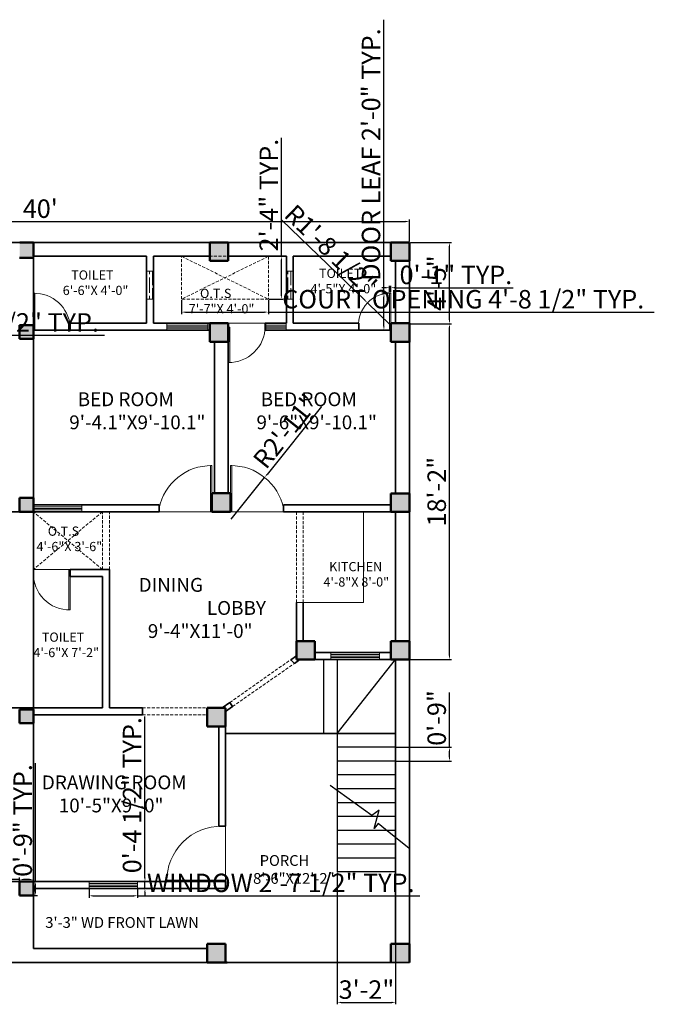
# Model space of a CAD drawing. Units: inches. Extents: x 2499 to 3266, y 1908 to 2597.
# Tile 2 of 2: x 2854 to 3266, y 1956 to 2597. Entities that reach past the tile are written whole.
import ezdxf

# ---------------------------------------------------------------- set-up
doc = ezdxf.new("R2010")
doc.units = ezdxf.units.IN
doc.linetypes.add('JIS_02_2.0', pattern=[3, 2, -1])
for name, color, linetype, lineweight in [('A-ANNO-DIMS', 2, 'Continuous', 18), ('A-AREA-IDEN', 7, 'Continuous', 18), ('A-COLS', 7, 'Continuous', 50), ('A-FLOR-FIXT', 9, 'Continuous', 18), ('A-FLOR-OPEN', 6, 'JIS_02_2.0', 13), ('A-FLOR-STRS', 7, 'Continuous', 25), ('A-GLAZ', 5, 'Continuous', 18), ('A-GLAZ-PATT', 4, 'Continuous', 13), ('A-WALL', 7, 'Continuous', 35), ('A-WALL-OVHD', 6, 'JIS_02_2.0', 18)]:
    doc.layers.add(name, color=color, linetype=linetype, lineweight=lineweight)
doc.layers.add('A-COLS-PATT', color=177, linetype='Continuous', lineweight=13, true_color=0x293189)
doc.layers.add('A-DOOR', color=32, linetype='Continuous', lineweight=18, true_color=0xcd6928)
doc.styles.get("Standard").update_dxf_attribs({"font": 'arial.ttf'})
doc.dimstyles.new('ISO-25', dxfattribs={"dimtxt": 12, "dimasz": 2.5, "dimexe": 1.25, "dimexo": 0.625, "dimtad": 1, "dimdec": 1, "dimlunit": 3, "dimtxsty": 'Standard', "dimcen": 2.5, "dimadec": 0, "dimazin": 0, "dimtfac": 1, "dimtdec": 1, "dimtmove": 0, "dimatfit": 3, "dimfxl": 1, "dimarcsym": 0})

# ---------------------------------------------------------------- blocks, each defined once
blk = doc.blocks.new('*D4')
at = {"layer": 'A-ANNO-DIMS', "color": 0, "lineweight": -2, "transparency": 16777216}
for p, q in [((2627.06, 2452.33), (2627.06, 2466.64)), ((2629.56, 2465.39), (3104.56, 2465.39)), ((3107.06, 2452.33), (3107.06, 2466.64))]:
    blk.add_line(p, q, dxfattribs=at)
at = {"layer": 'A-ANNO-DIMS', "color": 0, "transparency": 16777216}
for points in [[(2629.56, 2465.81), (2629.56, 2464.98), (2627.06, 2465.39)], [(3104.56, 2465.81), (3104.56, 2464.98), (3107.06, 2465.39)]]:
    blk.add_solid(points, dxfattribs=at)
at = {"layer": 'Defpoints', "color": 0, "transparency": 16777216}
for p in [(3107.06, 2465.39), (2627.06, 2451.71), (3107.06, 2451.71)]:
    blk.add_point(p, dxfattribs=at)
at = {"layer": 'A-ANNO-DIMS', "color": 0, "transparency": 16777216, "insert": (2867.06, 2472.14), "char_height": 12, "attachment_point": 5}
blk.add_mtext("40'", dxfattribs=at)
blk = doc.blocks.new('COL-12X12')
for p, q in [((0, 12), (12, 12)), ((0, 0), (0, 12)), ((12, 12), (12, 0)), ((12, 0), (0, 0))]:
    blk.add_line(p, q)
blk = doc.blocks.new('COL-9X9')
for p, q in [((0, 9), (9, 9)), ((0, 0), (0, 9)), ((9, 9), (9, 0)), ((9, 0), (0, 0))]:
    blk.add_line(p, q)
blk = doc.blocks.new('WIN-31_54')
for p, q in [((0, 4.5), (0, 0)), ((0, 3.25), (31.54, 3.25)), ((0, 2.25), (31.54, 2.25)), ((0, 1.25), (31.54, 1.25)), ((31.54, 0), (31.54, 4.5)), ((31.54, 3.25), (31.54, 0))]:
    blk.add_line(p, q)
blk = doc.blocks.new('STAIR-BREAK')
for p, q in [((28.01, 16.3), (55.25, 35.7)), ((16.69, 10.65), (21.73, 13.87)), ((21.73, 13.87), (19.46, 17.43)), ((19.46, 17.43), (29.77, 10.65)), ((29.77, 10.65), (28.01, 16.3)), ((0, 0), (16.69, 10.65))]:
    blk.add_line(p, q)
blk = doc.blocks.new('OTS-REAR-OPENING')
for p, q in [((0, 27.82), (56.41, 0)), ((56.41, 27.82), (0, 0))]:
    blk.add_line(p, q)
blk.add_lwpolyline([(0, 27.82), (56.41, 27.82), (56.41, 0), (0, 0)], close=True)
blk = doc.blocks.new('DOOR-LEAF-24')
for p, q in [((0, 0), (0, 24)), ((0, 24), (1, 24)), ((1, 24), (1, 0)), ((1, 0), (0, 0))]:
    blk.add_line(p, q)
blk = doc.blocks.new('DOOR-LEAF-30')
for p, q in [((0, 6), (0, 30)), ((0, 30), (1, 30)), ((1, 30), (1, 0)), ((1, 0), (0, 0))]:
    blk.add_line(p, q)
blk = doc.blocks.new('*D16')
at = {"layer": 'A-ANNO-DIMS', "color": 0, "lineweight": -2, "transparency": 16777216}
for p, q in [((2853.56, 2037.57), (2589.1, 2037.57)), ((2853.56, 2036.85), (2853.56, 2038.82)), ((2860.06, 2037.57), (2856.06, 2037.57)), ((2862.56, 2036.85), (2862.56, 2038.82))]:
    blk.add_line(p, q, dxfattribs=at)
at = {"layer": 'A-ANNO-DIMS', "color": 0, "transparency": 16777216}
for points in [[(2856.06, 2037.99), (2856.06, 2037.15), (2853.56, 2037.57)], [(2860.06, 2037.99), (2860.06, 2037.15), (2862.56, 2037.57)]]:
    blk.add_solid(points, dxfattribs=at)
at = {"layer": 'Defpoints', "color": 0, "transparency": 16777216}
for p in [(2853.56, 2037.57), (2853.56, 2036.22), (2862.56, 2036.22)]:
    blk.add_point(p, dxfattribs=at)
at = {"layer": 'A-ANNO-DIMS', "color": 0, "transparency": 16777216, "insert": (2720.08, 2044.4), "char_height": 12, "attachment_point": 5}
blk.add_mtext('PARTY WALL COLUMN 0\'-9" TYP.', dxfattribs=at)
blk = doc.blocks.new('*D17')
at = {"layer": 'A-ANNO-DIMS', "color": 0, "lineweight": -2, "transparency": 16777216}
for p, q in [((2863.91, 2036.22), (2863.91, 2113.12)), ((2863.18, 2036.22), (2865.16, 2036.22)), ((2863.91, 2029.72), (2863.91, 2033.72)), ((2863.18, 2027.22), (2865.16, 2027.22))]:
    blk.add_line(p, q, dxfattribs=at)
at = {"layer": 'A-ANNO-DIMS', "color": 0, "transparency": 16777216}
for points in [[(2863.49, 2033.72), (2864.32, 2033.72), (2863.91, 2036.22)], [(2863.49, 2029.72), (2864.32, 2029.72), (2863.91, 2027.22)]]:
    blk.add_solid(points, dxfattribs=at)
at = {"layer": 'Defpoints', "color": 0, "transparency": 16777216}
for p in [(2862.56, 2036.22), (2863.91, 2036.22), (2862.56, 2027.22)]:
    blk.add_point(p, dxfattribs=at)
at = {"layer": 'A-ANNO-DIMS', "color": 0, "transparency": 16777216, "insert": (2857.16, 2075.92), "char_height": 12, "attachment_point": 5, "rotation": 90}
blk.add_mtext('0\'-9" TYP.', dxfattribs=at)
blk = doc.blocks.new('*D18')
at = {"layer": 'A-ANNO-DIMS', "color": 0, "lineweight": -2, "transparency": 16777216}
for p, q in [((2898.81, 2031.08), (2898.81, 2025.73)), ((2930.35, 2031.08), (2930.35, 2025.73)), ((2901.31, 2026.98), (2927.85, 2026.98)), ((2930.35, 2026.98), (3113.91, 2026.98))]:
    blk.add_line(p, q, dxfattribs=at)
at = {"layer": 'A-ANNO-DIMS', "color": 0, "transparency": 16777216}
for points in [[(2901.31, 2027.39), (2901.31, 2026.56), (2898.81, 2026.98)], [(2927.85, 2027.39), (2927.85, 2026.56), (2930.35, 2026.98)]]:
    blk.add_solid(points, dxfattribs=at)
at = {"layer": 'Defpoints', "color": 0, "transparency": 16777216}
for p in [(2898.81, 2031.71), (2930.35, 2031.71), (2930.35, 2026.98)]:
    blk.add_point(p, dxfattribs=at)
at = {"layer": 'A-ANNO-DIMS', "color": 0, "transparency": 16777216, "insert": (3023.38, 2033.81), "char_height": 12, "attachment_point": 5}
blk.add_mtext('WINDOW 2\'-7 1/2" TYP.', dxfattribs=at)
blk = doc.blocks.new('*D19')
at = {"layer": 'A-ANNO-DIMS', "color": 0, "lineweight": -2, "transparency": 16777216}
for p, q in [((2935.08, 2038.71), (2935.08, 2143.57)), ((2930.97, 2036.21), (2936.33, 2036.21)), ((2935.08, 2031.71), (2935.08, 2036.21)), ((2930.97, 2031.71), (2936.33, 2031.71)), ((2935.08, 2029.21), (2935.08, 2026.71))]:
    blk.add_line(p, q, dxfattribs=at)
at = {"layer": 'A-ANNO-DIMS', "color": 0, "transparency": 16777216}
for points in [[(2934.66, 2038.71), (2935.5, 2038.71), (2935.08, 2036.21)], [(2934.66, 2029.21), (2935.5, 2029.21), (2935.08, 2031.71)]]:
    blk.add_solid(points, dxfattribs=at)
at = {"layer": 'Defpoints', "color": 0, "transparency": 16777216}
for p in [(2930.35, 2036.21), (2935.08, 2036.21), (2930.35, 2031.71)]:
    blk.add_point(p, dxfattribs=at)
at = {"layer": 'A-ANNO-DIMS', "color": 0, "transparency": 16777216, "insert": (2928.25, 2092.39), "char_height": 12, "attachment_point": 5, "rotation": 90}
blk.add_mtext('0\'-4 1/2" TYP.', dxfattribs=at)
blk = doc.blocks.new('*D20')
at = {"layer": 'A-ANNO-DIMS', "color": 0, "lineweight": -2, "transparency": 16777216}
for p, q in [((2693.56, 2394.08), (2693.56, 2390.1)), ((2715.97, 2394.08), (2715.97, 2390.1)), ((2696.06, 2391.35), (2713.47, 2391.35)), ((2715.97, 2391.35), (2908.86, 2391.35))]:
    blk.add_line(p, q, dxfattribs=at)
at = {"layer": 'A-ANNO-DIMS', "color": 0, "transparency": 16777216}
for points in [[(2696.06, 2391.76), (2696.06, 2390.93), (2693.56, 2391.35)], [(2713.47, 2391.76), (2713.47, 2390.93), (2715.97, 2391.35)]]:
    blk.add_solid(points, dxfattribs=at)
at = {"layer": 'Defpoints', "color": 0, "transparency": 16777216}
for p in [(2693.56, 2394.71), (2715.97, 2394.71), (2715.97, 2391.35)]:
    blk.add_point(p, dxfattribs=at)
at = {"layer": 'A-ANNO-DIMS', "color": 0, "transparency": 16777216, "insert": (2813.66, 2398.18), "char_height": 12, "attachment_point": 5}
blk.add_mtext('WINDOW 1\'-10 1/2" TYP.', dxfattribs=at)
blk = doc.blocks.new('*D22')
at = {"layer": 'A-ANNO-DIMS', "color": 0, "lineweight": -2, "transparency": 16777216}
for p, q in [((3090.46, 2418.71), (3090.46, 2596.54)), ((3093.43, 2418.71), (3089.21, 2418.71)), ((3090.46, 2397.21), (3090.46, 2416.21)), ((3093.43, 2394.71), (3089.21, 2394.71))]:
    blk.add_line(p, q, dxfattribs=at)
at = {"layer": 'A-ANNO-DIMS', "color": 0, "transparency": 16777216}
for points in [[(3090.04, 2416.21), (3090.87, 2416.21), (3090.46, 2418.71)], [(3090.04, 2397.21), (3090.87, 2397.21), (3090.46, 2394.71)]]:
    blk.add_solid(points, dxfattribs=at)
at = {"layer": 'Defpoints', "color": 0, "transparency": 16777216}
for p in [(3090.46, 2418.71), (3094.06, 2418.71), (3094.06, 2394.71)]:
    blk.add_point(p, dxfattribs=at)
at = {"layer": 'A-ANNO-DIMS', "color": 0, "transparency": 16777216, "insert": (3083.62, 2508.87), "char_height": 12, "attachment_point": 5, "rotation": 90}
blk.add_mtext('DOOR LEAF 2\'-0" TYP.', dxfattribs=at)
blk = doc.blocks.new('*D23')
at = {"layer": 'A-ANNO-DIMS', "color": 0, "lineweight": -2, "transparency": 16777216}
for p, q in [((3091.56, 2422.31), (3089.06, 2422.31)), ((3094.06, 2419.33), (3094.06, 2423.56)), ((3094.06, 2422.31), (3095.06, 2422.31)), ((3095.06, 2419.33), (3095.06, 2423.56)), ((3097.56, 2422.31), (3174.45, 2422.31))]:
    blk.add_line(p, q, dxfattribs=at)
at = {"layer": 'A-ANNO-DIMS', "color": 0, "transparency": 16777216}
for points in [[(3091.56, 2422.73), (3091.56, 2421.89), (3094.06, 2422.31)], [(3097.56, 2422.73), (3097.56, 2421.89), (3095.06, 2422.31)]]:
    blk.add_solid(points, dxfattribs=at)
at = {"layer": 'Defpoints', "color": 0, "transparency": 16777216}
for p in [(3095.06, 2422.31), (3094.06, 2418.71), (3095.06, 2418.71)]:
    blk.add_point(p, dxfattribs=at)
at = {"layer": 'A-ANNO-DIMS', "color": 0, "transparency": 16777216, "insert": (3137.25, 2429.06), "char_height": 12, "attachment_point": 5}
blk.add_mtext('0\'-1" TYP.', dxfattribs=at)
blk = doc.blocks.new('*D26')
at = {"layer": 'A-ANNO-DIMS', "color": 0, "lineweight": -2, "transparency": 16777216}
for p, q in [((2958.91, 2414.26), (2958.91, 2405.17)), ((3015.32, 2414.26), (3015.32, 2405.17)), ((2961.41, 2406.42), (3012.82, 2406.42)), ((3015.32, 2406.42), (3266.27, 2406.42))]:
    blk.add_line(p, q, dxfattribs=at)
at = {"layer": 'A-ANNO-DIMS', "color": 0, "transparency": 16777216}
for points in [[(2961.41, 2406.84), (2961.41, 2406.01), (2958.91, 2406.42)], [(3012.82, 2406.84), (3012.82, 2406.01), (3015.32, 2406.42)]]:
    blk.add_solid(points, dxfattribs=at)
at = {"layer": 'Defpoints', "color": 0, "transparency": 16777216}
for p in [(2958.91, 2414.89), (3015.32, 2414.89), (3015.32, 2406.42)]:
    blk.add_point(p, dxfattribs=at)
at = {"layer": 'A-ANNO-DIMS', "color": 0, "transparency": 16777216, "insert": (3142.04, 2413.26), "char_height": 12, "attachment_point": 5}
blk.add_mtext('COURT OPENING 4\'-8 1/2" TYP.', dxfattribs=at)
blk = doc.blocks.new('*D27')
at = {"layer": 'A-ANNO-DIMS', "color": 0, "lineweight": -2, "transparency": 16777216}
for p, q in [((3023.78, 2442.71), (3023.78, 2519.81)), ((3015.95, 2442.71), (3025.03, 2442.71)), ((3023.78, 2417.39), (3023.78, 2440.21)), ((3015.95, 2414.89), (3025.03, 2414.89))]:
    blk.add_line(p, q, dxfattribs=at)
at = {"layer": 'A-ANNO-DIMS', "color": 0, "transparency": 16777216}
for points in [[(3023.37, 2440.21), (3024.2, 2440.21), (3023.78, 2442.71)], [(3023.37, 2417.39), (3024.2, 2417.39), (3023.78, 2414.89)]]:
    blk.add_solid(points, dxfattribs=at)
at = {"layer": 'Defpoints', "color": 0, "transparency": 16777216}
for p in [(3015.32, 2442.71), (3023.78, 2442.71), (3015.32, 2414.89)]:
    blk.add_point(p, dxfattribs=at)
at = {"layer": 'A-ANNO-DIMS', "color": 0, "transparency": 16777216, "insert": (3017.13, 2482.51), "char_height": 12, "attachment_point": 5, "rotation": 90}
blk.add_mtext('2\'-4" TYP.', dxfattribs=at)
blk = doc.blocks.new('*D29')
at = {"layer": 'A-ANNO-DIMS', "color": 0, "lineweight": -2, "transparency": 16777216}
for p, q in [((3107.68, 2398.84), (3134.33, 2398.84)), ((3133.08, 2183.11), (3133.08, 2396.34)), ((3107.68, 2180.61), (3134.33, 2180.61))]:
    blk.add_line(p, q, dxfattribs=at)
at = {"layer": 'A-ANNO-DIMS', "color": 0, "transparency": 16777216}
for points in [[(3132.67, 2396.34), (3133.5, 2396.34), (3133.08, 2398.84)], [(3132.67, 2183.11), (3133.5, 2183.11), (3133.08, 2180.61)]]:
    blk.add_solid(points, dxfattribs=at)
at = {"layer": 'Defpoints', "color": 0, "transparency": 16777216}
for p in [(3107.06, 2398.84), (3133.08, 2398.84), (3107.06, 2180.61)]:
    blk.add_point(p, dxfattribs=at)
at = {"layer": 'A-ANNO-DIMS', "color": 0, "transparency": 16777216, "insert": (3126.33, 2289.72), "char_height": 12, "attachment_point": 5, "rotation": 90}
blk.add_mtext('18\'-2"', dxfattribs=at)
blk = doc.blocks.new('*D30')
at = {"layer": 'A-ANNO-DIMS', "color": 0, "lineweight": -2, "transparency": 16777216}
for p, q in [((3107.68, 2451.71), (3134.33, 2451.71)), ((3133.08, 2401.34), (3133.08, 2449.21)), ((3107.68, 2398.84), (3134.33, 2398.84))]:
    blk.add_line(p, q, dxfattribs=at)
at = {"layer": 'A-ANNO-DIMS', "color": 0, "transparency": 16777216}
for points in [[(3132.67, 2449.21), (3133.5, 2449.21), (3133.08, 2451.71)], [(3132.67, 2401.34), (3133.5, 2401.34), (3133.08, 2398.84)]]:
    blk.add_solid(points, dxfattribs=at)
at = {"layer": 'Defpoints', "color": 0, "transparency": 16777216}
for p in [(3107.06, 2451.71), (3133.08, 2451.71), (3107.06, 2398.84)]:
    blk.add_point(p, dxfattribs=at)
at = {"layer": 'A-ANNO-DIMS', "color": 0, "transparency": 16777216, "insert": (3126.35, 2425.27), "char_height": 12, "attachment_point": 5, "rotation": 90}
blk.add_mtext('4\'-5"', dxfattribs=at)
blk = doc.blocks.new('*D32')
at = {"layer": 'A-ANNO-DIMS', "color": 0, "lineweight": -2, "transparency": 16777216}
for p, q in [((3060.16, 2041.89), (3060.16, 1956.43)), ((3098.06, 2041.89), (3098.06, 1956.43)), ((3062.66, 1957.68), (3095.56, 1957.68))]:
    blk.add_line(p, q, dxfattribs=at)
at = {"layer": 'A-ANNO-DIMS', "color": 0, "transparency": 16777216}
for points in [[(3062.66, 1958.1), (3062.66, 1957.27), (3060.16, 1957.68)], [(3095.56, 1958.1), (3095.56, 1957.27), (3098.06, 1957.68)]]:
    blk.add_solid(points, dxfattribs=at)
at = {"layer": 'Defpoints', "color": 0, "transparency": 16777216}
for p in [(3060.16, 2042.51), (3098.06, 2042.51), (3098.06, 1957.68)]:
    blk.add_point(p, dxfattribs=at)
at = {"layer": 'A-ANNO-DIMS', "color": 0, "transparency": 16777216, "insert": (3079.11, 1964.44), "char_height": 12, "attachment_point": 5}
blk.add_mtext('3\'-2"', dxfattribs=at)
blk = doc.blocks.new('*D33')
at = {"layer": 'A-ANNO-DIMS', "color": 0, "lineweight": -2, "transparency": 16777216}
for p, q in [((3133.08, 2123.51), (3133.08, 2159.16)), ((3098.68, 2123.51), (3134.33, 2123.51)), ((3133.08, 2117.01), (3133.08, 2121.01)), ((3098.68, 2114.51), (3134.33, 2114.51))]:
    blk.add_line(p, q, dxfattribs=at)
at = {"layer": 'A-ANNO-DIMS', "color": 0, "transparency": 16777216}
for points in [[(3132.67, 2121.01), (3133.5, 2121.01), (3133.08, 2123.51)], [(3132.67, 2117.01), (3133.5, 2117.01), (3133.08, 2114.51)]]:
    blk.add_solid(points, dxfattribs=at)
at = {"layer": 'Defpoints', "color": 0, "transparency": 16777216}
for p in [(3098.06, 2123.51), (3133.08, 2123.51), (3098.06, 2114.51)]:
    blk.add_point(p, dxfattribs=at)
at = {"layer": 'A-ANNO-DIMS', "color": 0, "transparency": 16777216, "insert": (3126.33, 2142.58), "char_height": 12, "attachment_point": 5, "rotation": 90}
blk.add_mtext('0\'-9"', dxfattribs=at)
blk = doc.blocks.new('*D35')
at = {"layer": 'A-ANNO-DIMS', "color": 0, "lineweight": -2, "transparency": 16777216}
for p, q in [((3049.79, 2344.97), (3014.48, 2300.92)), ((2991.11, 2271.75), (3012.92, 2298.97))]:
    blk.add_line(p, q, dxfattribs=at)
at = {"layer": 'A-ANNO-DIMS', "color": 0, "transparency": 16777216}
blk.add_solid([(3014.16, 2301.18), (3014.81, 2300.66), (3012.92, 2298.97)], dxfattribs=at)
at = {"layer": 'Defpoints', "color": 0, "transparency": 16777216}
for p in [(3012.92, 2298.97), (2991.11, 2271.75)]:
    blk.add_point(p, dxfattribs=at)
at = {"layer": 'A-ANNO-DIMS', "color": 0, "transparency": 16777216, "insert": (3027.73, 2328.08), "char_height": 12, "attachment_point": 5, "rotation": 51.29209}
blk.add_mtext('R2\'-11"', dxfattribs=at)
blk = doc.blocks.new('*D39')
at = {"layer": 'A-ANNO-DIMS', "color": 0, "lineweight": -2, "transparency": 16777216}
for p, q in [((3023.96, 2466.34), (3077.98, 2414.18)), ((3094.56, 2398.18), (3079.78, 2412.44))]:
    blk.add_line(p, q, dxfattribs=at)
at = {"layer": 'A-ANNO-DIMS', "color": 0, "transparency": 16777216}
blk.add_solid([(3078.27, 2414.48), (3077.7, 2413.88), (3079.78, 2412.44)], dxfattribs=at)
at = {"layer": 'Defpoints', "color": 0, "transparency": 16777216}
for p in [(3079.78, 2412.44), (3094.56, 2398.18)]:
    blk.add_point(p, dxfattribs=at)
at = {"layer": 'A-ANNO-DIMS', "color": 0, "transparency": 16777216, "insert": (3054.82, 2446.04), "char_height": 12, "attachment_point": 5, "rotation": 316.00453}
blk.add_mtext('R1\'-8 1/2"', dxfattribs=at)

msp = doc.modelspace()

# ---------------------------------------------------------------- hatches: boundary and pattern name
at = {"layer": 'A-COLS-PATT'}
h = msp.add_hatch(color=256, dxfattribs=at)
h.dxf.hatch_style = 1
h.paths.add_polyline_path([(2639.06, 2451.71), (2627.06, 2451.71), (2627.06, 2439.9), (2639.06, 2439.9)])
h.paths.add_polyline_path([(2639.06, 2408.96), (2627.06, 2408.96), (2627.06, 2396.96), (2639.06, 2396.96)])
h.paths.add_polyline_path([(2759.22, 2451.71), (2747.22, 2451.71), (2747.22, 2439.71), (2759.22, 2439.71)])
h.paths.add_polyline_path([(2862.56, 2451.71), (2853.74, 2451.71), (2853.56, 2451.71), (2853.56, 2441.73), (2853.74, 2441.73), (2853.74, 2441.73), (2862.56, 2441.73), (2862.56, 2442.71)])
h.paths.add_polyline_path([(2989.26, 2451.71), (2977.26, 2451.71), (2977.26, 2439.71), (2989.26, 2439.71)])
h.paths.add_polyline_path([(3107.06, 2451.71), (3095.06, 2451.71), (3095.06, 2439.71), (3107.06, 2439.71)])
h.paths.add_polyline_path([(3107.06, 2399.21), (3095.06, 2399.21), (3095.06, 2387.21), (3107.06, 2387.21)])
h.paths.add_polyline_path([(2989.26, 2399.21), (2977.26, 2399.21), (2977.26, 2387.21), (2989.26, 2387.21)])
h.paths.add_polyline_path([(2862.56, 2397.96), (2853.56, 2397.96), (2853.56, 2388.96), (2862.56, 2388.96)])
h.paths.add_polyline_path([(2753.06, 2399.21), (2741.06, 2399.21), (2741.06, 2387.39), (2753.06, 2387.39)])
h.paths.add_polyline_path([(2639.06, 2288.56), (2627.06, 2288.56), (2627.06, 2276.56), (2636.06, 2276.56), (2636.06, 2276.61), (2639.06, 2276.61)])
h.paths.add_polyline_path([(2862.56, 2285.61), (2853.56, 2285.61), (2853.56, 2276.61), (2862.56, 2276.61)])
h.paths.add_polyline_path([(2990.61, 2288.63), (2978.61, 2288.63), (2978.61, 2276.63), (2990.61, 2276.63)])
h.paths.add_polyline_path([(3107.06, 2288.61), (3095.06, 2288.61), (3095.06, 2276.61), (3107.06, 2276.61)])
h.paths.add_polyline_path([(3107.06, 2192.61), (3095.06, 2192.61), (3095.06, 2180.61), (3107.06, 2180.61)])
h.paths.add_polyline_path([(3045.56, 2192.61), (3033.56, 2192.61), (3033.56, 2180.61), (3045.56, 2180.61)])
h.paths.add_polyline_path([(2639.06, 2192.61), (2627.06, 2192.61), (2627.06, 2180.61), (2639.06, 2180.61)])
h.paths.add_polyline_path([(2696.54, 2192.61), (2684.54, 2192.61), (2684.54, 2180.61), (2696.54, 2180.61)])
h.paths.add_polyline_path([(2740.56, 2149.11), (2728.56, 2149.11), (2728.56, 2137.17), (2740.56, 2137.17)])
h.paths.add_polyline_path([(2862.56, 2148.12), (2853.56, 2148.12), (2853.56, 2139.12), (2862.56, 2139.12)])
h.paths.add_polyline_path([(2987.56, 2149.11), (2975.54, 2149.11), (2975.54, 2137.05), (2987.56, 2137.05)])
h.paths.add_polyline_path([(2862.56, 2036.21), (2853.56, 2036.21), (2853.56, 2027.22), (2862.56, 2027.22)])
h.paths.add_polyline_path([(2639.06, 1995.71), (2627.06, 1995.71), (2627.06, 1983.71), (2639.06, 1983.71)])
h.paths.add_polyline_path([(2740.56, 1995.71), (2728.56, 1995.71), (2728.56, 1983.71), (2740.56, 1983.71)])
h.paths.add_polyline_path([(2987.56, 1995.71), (2975.56, 1995.71), (2975.56, 1983.71), (2987.56, 1983.71)])
h.paths.add_polyline_path([(3107.06, 1995.71), (3095.06, 1995.71), (3095.06, 1983.71), (3107.06, 1983.71)])
at = {"layer": 'A-GLAZ-PATT'}
h = msp.add_hatch(dxfattribs=at)
h.set_pattern_fill('GOST_WOOD', color=256)
h.paths.add_polyline_path([(2693.56, 2432.95), (2689.06, 2432.95), (2689.06, 2414.75), (2693.56, 2414.75)])
h.paths.add_polyline_path([(2784.56, 2432.95), (2780.06, 2432.95), (2780.06, 2414.75), (2784.56, 2414.75)])
h.paths.add_polyline_path([(2940.56, 2432.95), (2936.06, 2432.95), (2936.06, 2414.75), (2940.56, 2414.75)])
h.paths.add_polyline_path([(3031.56, 2432.95), (3027.06, 2432.95), (3027.06, 2414.75), (3031.56, 2414.75)])

# ---------------------------------------------------------------- linework, layer by layer
at = {"layer": 'A-COLS'}
for p, q in [((2853.74, 2451.71), (2862.52, 2451.71)), ((2862.56, 2451.71), (2853.74, 2451.71)), ((2862.56, 2442.71), (2862.56, 2451.71)), ((2977.26, 2439.71), (2977.26, 2451.71)), ((2853.74, 2441.73), (2853.56, 2441.73)), ((2853.74, 2441.73), (2862.56, 2441.73)), ((3107.06, 2398.84), (3107.06, 2386.84)), ((3098.06, 2192.61), (3107.06, 2192.61)), ((2975.54, 2137.05), (2975.54, 2149.11)), ((2975.55, 2149.11), (2987.55, 2149.11)), ((2987.56, 2149.05), (2987.56, 2137.05)), ((2987.54, 2137.05), (2975.54, 2137.05)), ((2987.56, 1995.71), (2987.56, 1983.71)), ((2987.56, 1992.71), (2987.56, 1992.71)), ((2987.56, 1992.71), (2987.56, 1983.71)), ((3107.06, 1995.71), (3095.06, 1995.71)), ((3095.06, 1995.71), (3095.06, 1983.71)), ((3107.06, 1983.71), (3107.06, 1995.71)), ((2988.58, 1983.71), (2976.58, 1983.71))]:
    msp.add_line(p, q, dxfattribs=at)
at = {"layer": 'A-DOOR'}
for p, q in [((2863.56, 2394.71), (2886.56, 2394.71)), ((2989.26, 2399.21), (2989.26, 2397.71)), ((3013.26, 2399.21), (2989.26, 2399.21)), ((2989.26, 2397.71), (2989.26, 2373.71)), ((2990.26, 2396.56), (2989.26, 2396.56)), ((2990.26, 2373.71), (2990.26, 2396.56)), ((3074.06, 2396.96), (3074.06, 2394.71)), ((3074.06, 2394.71), (3095.06, 2394.71)), ((2989.26, 2373.71), (2990.26, 2373.71)), ((2977.61, 2276.63), (2944.26, 2276.63)), ((2990.61, 2276.63), (3025.26, 2276.61)), ((2885.56, 2239.11), (2862.56, 2239.11)), ((2885.56, 2212.86), (2885.56, 2239.11)), ((2885.56, 2239.11), (2886.56, 2239.11)), ((2886.56, 2236.86), (2886.56, 2212.86)), ((2886.56, 2212.86), (2885.56, 2212.86)), ((2987.56, 2037.21), (2987.56, 2072.21)), ((2949.26, 2036.21), (2949.26, 2037.21)), ((2949.26, 2037.21), (2987.56, 2037.21)), ((2961.26, 2036.21), (2949.26, 2036.21)), ((2985.26, 2036.21), (2961.26, 2036.21)), ((2987.56, 2037.21), (2987.56, 2036.21))]:
    msp.add_line(p, q, dxfattribs=at)
for centre, radius, start, end in [((2863.06, 2395.14), 23.57, 4.41558, 91.21553), ((3094.56, 2398.18), 20.54, 88.60487, 183.4053), ((2989.76, 2397.2), 23.5, 268.78092, 359.40032), ((2978.11, 2272.11), 34.52, 89.16997, 168.73212), ((2991.11, 2271.75), 34.88, 11.76226, 90.82131), ((2886.06, 2236.37), 23.51, 178.08221, 271.21847), ((2984.76, 2036.71), 35.5, 89.11918, 180.80691)]:
    msp.add_arc(centre, radius, start, end, dxfattribs=at)
at = {"layer": 'A-FLOR-FIXT'}
for p, q in [((3077.14, 2276.61), (3077.14, 2217.63)), ((3077.14, 2217.63), (3033.56, 2217.63))]:
    msp.add_line(p, q, dxfattribs=at)
at = {"layer": 'A-FLOR-OPEN'}
for p, q in [((2907.4, 2239.11), (2862.56, 2276.61)), ((2907.4, 2276.61), (2862.56, 2239.11)), ((2907.4, 2239.11), (2907.4, 2276.61)), ((2912.06, 2239.11), (2912.06, 2276.61))]:
    msp.add_line(p, q, dxfattribs=at)
at = {"layer": 'A-FLOR-STRS'}
for p, q in [((3051.16, 2180.61), (3051.16, 2132.51)), ((3060.16, 2180.61), (3060.16, 2042.51)), ((3060.16, 2180.61), (3069.16, 2180.61)), ((3060.16, 2132.51), (3098.06, 2180.61)), ((2987.56, 2132.51), (3098.06, 2132.51)), ((3098.06, 2132.51), (2987.56, 2132.51)), ((3098.06, 2132.51), (3098.06, 2123.51)), ((3098.06, 2123.51), (3060.16, 2123.51)), ((3098.06, 2114.51), (3060.16, 2114.51)), ((3098.06, 2105.51), (3060.16, 2105.51)), ((3098.06, 2096.51), (3060.16, 2096.51)), ((3098.06, 2087.51), (3060.16, 2087.51)), ((3098.06, 2078.51), (3060.16, 2078.51)), ((3098.06, 2069.51), (3060.16, 2069.51)), ((3098.06, 2060.51), (3060.16, 2060.51)), ((3098.06, 2051.51), (3060.16, 2051.51)), ((3098.06, 2042.51), (3060.16, 2042.51))]:
    msp.add_line(p, q, dxfattribs=at)
at = {"layer": 'A-GLAZ'}
for p, q in [((2936.06, 2432.95), (2940.56, 2432.95)), ((3027.06, 2432.95), (3031.56, 2432.95)), ((2936.06, 2414.75), (2940.56, 2414.75)), ((3027.06, 2414.75), (3031.56, 2414.75)), ((2949.3, 2399.21), (2949.3, 2394.71)), ((2976.02, 2397.96), (2949.3, 2397.96)), ((2976.02, 2396.96), (2949.3, 2396.96)), ((2976.02, 2395.96), (2949.3, 2395.96)), ((2976.02, 2399.21), (2976.02, 2394.71)), ((3013.59, 2399.21), (3013.59, 2394.71)), ((3026.87, 2397.96), (3013.59, 2397.96)), ((3026.87, 2396.96), (3013.59, 2396.96)), ((3026.87, 2395.96), (3013.59, 2395.96)), ((3026.87, 2399.21), (3026.87, 2394.71))]:
    msp.add_line(p, q, dxfattribs=at)
at = {"layer": 'A-WALL'}
for p, q in [((2627.06, 2451.71), (3107.06, 2451.71)), ((3107.06, 2451.71), (3107.06, 1983.71)), ((2862.56, 1992.71), (2862.56, 2442.71)), ((2862.56, 2442.71), (2936.06, 2442.71)), ((2936.06, 2399.21), (2936.06, 2442.71)), ((2940.56, 2399.21), (2940.56, 2442.71)), ((2940.56, 2442.71), (2977.26, 2442.71)), ((2989.26, 2442.71), (3027.06, 2442.71)), ((3027.06, 2399.21), (3027.06, 2442.71)), ((3031.56, 2399.21), (3031.56, 2442.71)), ((3031.56, 2442.71), (3095.06, 2442.71)), ((3098.06, 2439.71), (3098.06, 2399.21)), ((2862.56, 2394.71), (2886.56, 2394.71)), ((2886.56, 2394.71), (2886.56, 2399.21)), ((2886.56, 2399.21), (2936.06, 2399.21)), ((2886.56, 2394.71), (2977.26, 2394.71)), ((2940.56, 2399.21), (2989.26, 2399.21)), ((2989.26, 2288.63), (2989.26, 2399.21)), ((3013.26, 2399.21), (3013.26, 2394.71)), ((3013.26, 2399.21), (3027.06, 2399.21)), ((3013.26, 2394.71), (3074.06, 2394.71)), ((3031.56, 2399.21), (3074.06, 2399.21)), ((3074.06, 2394.71), (3074.06, 2399.21)), ((3074.06, 2394.71), (3095.06, 2394.71)), ((2980.26, 2288.63), (2980.26, 2387.21)), ((3098.06, 2387.21), (3098.06, 2288.61)), ((2862.56, 2281.11), (2944.26, 2281.11)), ((2944.26, 2276.61), (2944.26, 2281.11)), ((3025.26, 2276.61), (3025.26, 2281.11)), ((3025.26, 2281.11), (3095.06, 2281.11)), ((2786.06, 2276.61), (2944.26, 2276.61)), ((2980.26, 2276.61), (2980.26, 2276.63)), ((2980.26, 2276.61), (2989.26, 2276.61)), ((2989.26, 2276.61), (2989.26, 2276.63)), ((2989.26, 2276.63), (2989.26, 2276.61)), ((3025.26, 2276.61), (3033.56, 2276.61)), ((3025.26, 2276.61), (3098.06, 2276.61)), ((3098.06, 2276.61), (3098.06, 2192.61)), ((2886.56, 2239.11), (2886.56, 2234.61)), ((2886.56, 2239.11), (2912.06, 2239.11)), ((2886.56, 2234.61), (2907.56, 2234.61)), ((2907.56, 2149.11), (2907.56, 2234.61)), ((2912.06, 2149.11), (2912.06, 2239.11)), ((3033.56, 2217.63), (3033.56, 2180.61)), ((3038.06, 2217.63), (3038.06, 2192.61)), ((3029.85, 2180.47), (3033.56, 2183.08)), ((3045.56, 2185.11), (3095.06, 2185.11)), ((3029.85, 2180.47), (3032.23, 2178.07)), ((3032.23, 2178.07), (3035.86, 2180.61)), ((3033.56, 2180.61), (3098.06, 2180.61)), ((3033.56, 2180.61), (3035.86, 2180.61)), ((3098.06, 2180.61), (3098.06, 1995.71)), ((2985.31, 2149.11), (2990.3, 2152.62)), ((2990.3, 2152.62), (2992.11, 2150.04)), ((2804.06, 2149.11), (2907.56, 2149.11)), ((2804.06, 2149.11), (2907.56, 2149.11)), ((2862.56, 2144.61), (2912.06, 2144.61)), ((2862.56, 2144.61), (2933.54, 2144.61)), ((2912.06, 2149.11), (2933.54, 2149.11)), ((2933.54, 2144.61), (2933.54, 2149.11)), ((2975.54, 2149.11), (2983.06, 2149.11)), ((2983.06, 2149.11), (2987.56, 2149.11)), ((2987.56, 2146.86), (2992.11, 2150.04)), ((2987.56, 2149.11), (2987.56, 2144.61)), ((2987.56, 2072.21), (2987.56, 2144.61)), ((2983.06, 2072.21), (2983.06, 2137.05)), ((2983.06, 2072.21), (2987.56, 2072.21)), ((2987.56, 2036.21), (2728.56, 2036.21)), ((2987.56, 2031.71), (2987.56, 2036.21)), ((2987.56, 2031.71), (2862.56, 2031.71)), ((2975.56, 1992.71), (2862.56, 1992.71)), ((3107.06, 1983.71), (2627.06, 1983.71))]:
    msp.add_line(p, q, dxfattribs=at)
at = {"layer": 'A-WALL-OVHD'}
for p, q in [((3033.56, 2217.63), (3033.56, 2276.61)), ((3038.06, 2217.63), (3038.06, 2276.61)), ((2990.3, 2152.62), (3029.85, 2180.47)), ((2992.11, 2150.04), (3032.23, 2178.07)), ((2933.54, 2149.11), (2975.55, 2149.11)), ((2933.54, 2144.61), (2975.54, 2144.61))]:
    msp.add_line(p, q, dxfattribs=at)

# ---------------------------------------------------------------- block references
at = {"layer": 'A-COLS'}
for name, p, rotation in [('COL-12X12', (2977.26, 2451.71), 270.0000000000043), ('COL-12X12', (3107.06, 2439.71), 90), ('COL-12X12', (2989.26, 2387.21), 90.00000000000435), ('COL-12X12', (3107.06, 2387.21), 90), ('COL-9X9', (2862.56, 2276.61), 89.9999999999884), ('COL-12X12', (2990.61, 2276.63), 90), ('COL-12X12', (3107.06, 2180.61), 90), ('COL-9X9', (2862.56, 2139.12), 89.99999999998552), ('COL-9X9', (2862.56, 2027.22), 89.99999999999422)]:
    msp.add_blockref(name, p, dxfattribs=dict(at, rotation=rotation))
for name, p in [('COL-9X9', (2853.56, 2388.96)), ('COL-12X12', (3095.06, 2276.61)), ('COL-12X12', (3033.56, 2180.61)), ('COL-12X12', (2975.56, 1983.71))]:
    msp.add_blockref(name, p, dxfattribs=at)
at = {"layer": 'A-DOOR', "rotation": 180}
msp.add_blockref('DOOR-LEAF-24', (2863.56, 2418.71), dxfattribs=at)
at = {"layer": 'A-DOOR'}
for name, p in [('DOOR-LEAF-24', (3094.06, 2394.71)), ('DOOR-LEAF-30', (2990.61, 2276.63))]:
    msp.add_blockref(name, p, dxfattribs=at)
at = {"layer": 'A-DOOR', "extrusion": (0, 0, -1), "zscale": -1}
msp.add_blockref('DOOR-LEAF-30', (-2978.61, 2276.63), dxfattribs=at)
at = {"layer": 'A-FLOR-OPEN'}
msp.add_blockref('OTS-REAR-OPENING', (2958.91, 2414.89), dxfattribs=at)
at = {"layer": 'A-FLOR-STRS', "rotation": 108.5388521035874}
msp.add_blockref('STAIR-BREAK', (3106.89, 2057.72), dxfattribs=at)
at = {"layer": 'A-GLAZ'}
for p in [(2862.56, 2276.61), (3056.03, 2180.61), (2898.81, 2031.71)]:
    msp.add_blockref('WIN-31_54', p, dxfattribs=at)

# ---------------------------------------------------------------- texts
at = {"layer": 'A-AREA-IDEN', "attachment_point": 1}
for s, width, insert, char_height in [('   TOILET \\P6\'-6"X 4\'-0"', 47.5104, (2881.63, 2433.55), 6), ('   TOILET \\P4\'-5"X 4\'-0"', 48.7877, (3042.76, 2434.65), 6), ('    O.T.S \\P7\'-7"X 4\'-0"', 47.5104, (2963.56, 2421.61), 6), ('  BED ROOM\\P9\'-4.1"X9\'-10.1"', 87.691, (2885.87, 2354.28), 9), ('  BED ROOM\\P 9\'-6"X9\'-10.1"', 87.691, (3004.84, 2354.28), 9), ('    O.T.S \\P4\'-6"X 3\'-6"', 47.5104, (2864.59, 2267.04), 6), ('  KITCHEN \\P4\'-8"X 8\'-0"', 44.2597, (3051.16, 2243.99), 6), ('\\pxqc;DINING                                 LOBBY\\P\\pql;   9\'-4"X11\'-0"', 87.691, (2928.71, 2233.61), 9), ('   TOILET \\P4\'-6"X 7\'-2"', 44.2597, (2862.56, 2198.13), 6), ('  DRAWING ROOM\\P      10\'-5"X9\'-0"', 122.0977, (2862.56, 2105.21), 9), ('  PORCH\\P8\'-6"X12\'-2"', 65.76, (3005.41, 2053.43), 7), ('3\'-3" WD FRONT LAWN', 110.856, (2870.31, 2013.14), 7)]:
    msp.add_mtext_dynamic_manual_height_columns(s, width=width, gutter_width=12.5, heights=[0], dxfattribs=dict(at, insert=insert, char_height=char_height))

# ---------------------------------------------------------------- dimensions: what is measured, and where the dimension line sits
at = {"layer": 'A-ANNO-DIMS'}
for base, p1, p2, angle, text, picture, middle in [((3090.46, 2418.71), (3094.06, 2394.71), (3094.06, 2418.71), 90, 'DOOR LEAF <> TYP.', '*D22', (3083.62, 2508.87)), ((3023.78, 2442.71), (3015.32, 2414.89), (3015.32, 2442.71), 90, '<> TYP.', '*D27', (3017.13, 2482.51)), ((2935.08, 2036.21), (2930.35, 2031.71), (2930.35, 2036.21), 90, '<> TYP.', '*D19', (2928.25, 2092.39)), ((2863.91, 2036.22), (2862.56, 2027.22), (2862.56, 2036.22), 90, '<> TYP.', '*D17', (2857.16, 2075.92)), ((2853.56, 2037.57), (2862.56, 2036.22), (2853.56, 2036.22), 180, 'PARTY WALL COLUMN <> TYP.', '*D16', (2720.08, 2044.4))]:
    dim = msp.add_linear_dim(base=base, p1=p1, p2=p2, angle=angle, text=text, dimstyle='ISO-25', override={"dimdec": 1, "dimlfac": 1, "dimrnd": 0, "dimzin": 1, "dimdsep": 46, "dimlunit": 4, "dimfrac": 2}, dxfattribs=at)
    dim.commit()
    dim.dimension.update_dxf_attribs({"geometry": picture, "text_midpoint": middle})
for base, p1, p2, override, picture, middle in [((3107.06, 2465.39), (2627.06, 2451.71), (3107.06, 2451.71), {"dimclrd": 0, "dimclre": 0, "dimclrt": 0}, '*D4', (2867.06, 2472.14)), ((3098.06, 1957.68), (3060.16, 2042.51), (3098.06, 2042.51), {"dimdec": 1, "dimlfac": 1, "dimrnd": 0, "dimzin": 1, "dimdsep": 46, "dimlunit": 4, "dimfrac": 2}, '*D32', (3079.11, 1964.44))]:
    dim = msp.add_linear_dim(base=base, p1=p1, p2=p2, dimstyle='ISO-25', override=override, dxfattribs=at)
    dim.commit()
    dim.dimension.update_dxf_attribs({"geometry": picture, "text_midpoint": middle})
for center, mpoint, picture, middle in [((3094.56, 2398.18), (3079.78, 2412.44), '*D39', (3054.82, 2446.04)), ((2991.11, 2271.75), (3012.92, 2298.97), '*D35', (3027.73, 2328.08))]:
    dim = msp.add_radius_dim(center=center, mpoint=mpoint, dimstyle='ISO-25', override={"dimdec": 1, "dimlfac": 1, "dimrnd": 0, "dimzin": 1, "dimdsep": 46, "dimlunit": 4, "dimfrac": 2}, dxfattribs=at)
    dim.commit()
    dim.dimension.update_dxf_attribs({"geometry": picture, "text_midpoint": middle})
for base, p1, p2, text, picture, middle in [((3015.32, 2406.42), (2958.91, 2414.89), (3015.32, 2414.89), 'COURT OPENING <> TYP.', '*D26', (3142.04, 2413.26)), ((3095.06, 2422.31), (3094.06, 2418.71), (3095.06, 2418.71), '<> TYP.', '*D23', (3137.25, 2429.06)), ((2715.97, 2391.35), (2693.56, 2394.71), (2715.97, 2394.71), 'WINDOW <> TYP.', '*D20', (2813.66, 2398.18)), ((2930.35, 2026.98), (2898.81, 2031.71), (2930.35, 2031.71), 'WINDOW <> TYP.', '*D18', (3023.38, 2033.81))]:
    dim = msp.add_linear_dim(base=base, p1=p1, p2=p2, text=text, dimstyle='ISO-25', override={"dimdec": 1, "dimlfac": 1, "dimrnd": 0, "dimzin": 1, "dimdsep": 46, "dimlunit": 4, "dimfrac": 2}, dxfattribs=at)
    dim.commit()
    dim.dimension.update_dxf_attribs({"geometry": picture, "text_midpoint": middle})
for base, p1, p2, picture, middle in [((3133.08, 2451.71), (3107.06, 2398.84), (3107.06, 2451.71), '*D30', (3126.35, 2425.27)), ((3133.08, 2398.84), (3107.06, 2180.61), (3107.06, 2398.84), '*D29', (3126.33, 2289.72)), ((3133.08, 2123.51), (3098.06, 2114.51), (3098.06, 2123.51), '*D33', (3126.33, 2142.58))]:
    dim = msp.add_linear_dim(base=base, p1=p1, p2=p2, angle=90, dimstyle='ISO-25', override={"dimdec": 1, "dimlfac": 1, "dimrnd": 0, "dimzin": 1, "dimdsep": 46, "dimlunit": 4, "dimfrac": 2}, dxfattribs=at)
    dim.commit()
    dim.dimension.update_dxf_attribs({"geometry": picture, "text_midpoint": middle})

doc.saveas('drawing.dxf')
